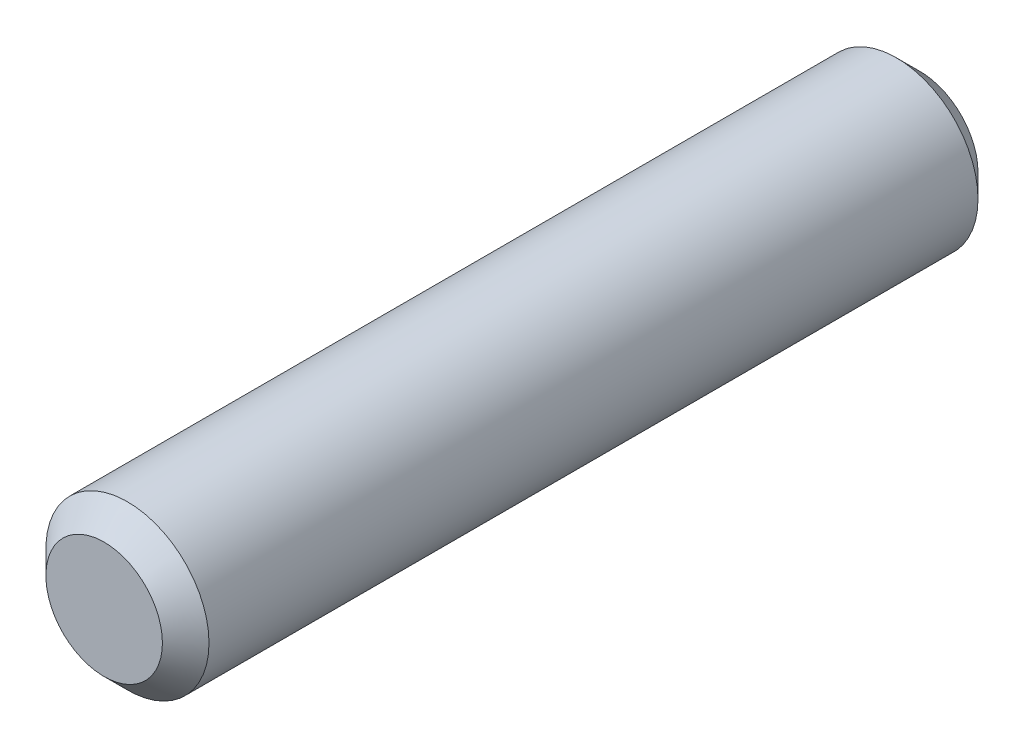
SolidWorks part; units mm, degrees
material "Plain Carbon Steel"
ref_plane "Front Plane" through (0, 0, 0) normal (0, 0, 1) x (1, 0, 0)
ref_plane "Top Plane" through (0, 0, 0) normal (0, 1, 0) x (1, 0, 0)
ref_plane "Right Plane" through (0, 0, 0) normal (1, 0, 0) x (0, 0, -1)
sketch "Pin Profile Ø14" plane through (0, 0, 0) normal (0, 0, 1) x (1, 0, 0)
  circle A0 centre (0, 0) radius 7
  dimension "D1" = 14
extrude "Pin Body Ø14x70" add sketch "Pin Profile Ø14" along normal mid plane 70
chamfer "End Chamfer 2x45 A" distance 2 angle 45 1 edges at (7, 0, 35)
chamfer "End Chamfer 2x45 B" distance 2 angle 45 1 edges at (7, 0, -35)
